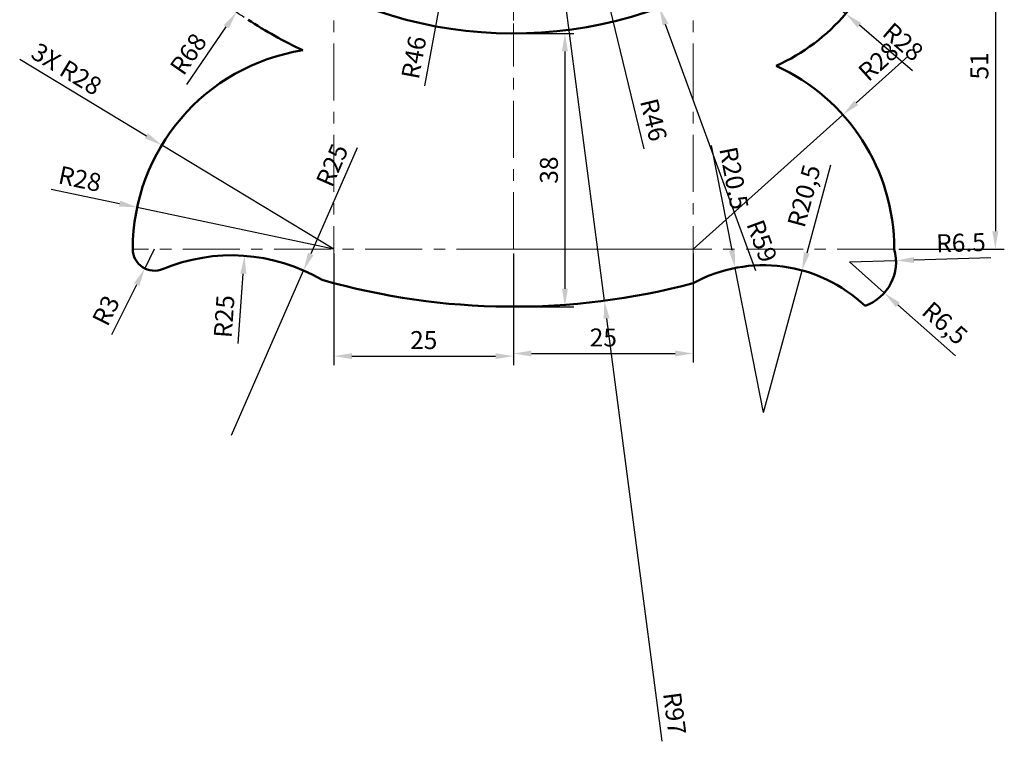
# Model space of a CAD drawing. Units: millimetres. Extents: x 2366 to 2507, y 1526 to 1734.
# Tile 1 of 2: x 2366 to 2503, y 1526 to 1627. Entities that reach past the tile are written whole.
import ezdxf

# ---------------------------------------------------------------- set-up
doc = ezdxf.new("R2010")
doc.units = ezdxf.units.MM
doc.linetypes.add('CENTER', pattern=[50.8, 31.75, -6.35, 6.35, -6.35])
for name, color, linetype, lineweight in [('M-CNTR', 4, 'CENTER', 18), ('M-DIMS', 2, 'Continuous', 25), ('M-OUTL', 7, 'Continuous', 50)]:
    doc.layers.add(name, color=color, linetype=linetype, lineweight=lineweight)
doc.styles.get("Standard").update_dxf_attribs({"font": 'arial.ttf'})
doc.dimstyles.new('ISO-25', dxfattribs={"dimtxt": 2.5, "dimasz": 2.5, "dimexe": 1.25, "dimexo": 0.625, "dimtad": 1, "dimtxsty": 'Standard', "dimcen": 2.5, "dimadec": 0, "dimazin": 0, "dimtfac": 1, "dimtmove": 0, "dimatfit": 3, "dimfxl": 1, "dimarcsym": 0})

# ---------------------------------------------------------------- blocks, each defined once
blk = doc.blocks.new('*D8')
at = {"layer": 'Defpoints', "color": 0, "transparency": 16777216}
for p in [(2492.86, 1645.78), (2488.16, 1594.78), (2502.23, 1594.78)]:
    blk.add_point(p, dxfattribs=at)
at = {"layer": 'M-DIMS', "color": 0, "lineweight": -2, "transparency": 16777216}
for p, q in [((2493.49, 1645.78), (2503.48, 1645.78)), ((2502.23, 1643.28), (2502.23, 1597.28)), ((2488.79, 1594.78), (2503.48, 1594.78))]:
    blk.add_line(p, q, dxfattribs=at)
at = {"layer": 'M-DIMS', "color": 0, "transparency": 16777216}
for points in [[(2501.81, 1643.28), (2502.64, 1643.28), (2502.23, 1645.78)], [(2501.81, 1597.28), (2502.64, 1597.28), (2502.23, 1594.78)]]:
    blk.add_solid(points, dxfattribs=at)
at = {"layer": 'M-DIMS', "color": 0, "transparency": 16777216, "insert": (2500.33, 1620.28), "char_height": 2.5, "attachment_point": 5, "rotation": 90}
blk.add_mtext('51', dxfattribs=at)
blk = doc.blocks.new('*D10')
at = {"layer": 'Defpoints', "color": 0, "transparency": 16777216}
for p in [(2410.16, 1594.78), (2435.16, 1594.78), (2435.16, 1579.9)]:
    blk.add_point(p, dxfattribs=at)
at = {"layer": 'M-DIMS', "color": 0, "lineweight": -2, "transparency": 16777216}
for p, q in [((2410.16, 1594.16), (2410.16, 1578.65)), ((2435.16, 1594.16), (2435.16, 1578.65)), ((2412.66, 1579.9), (2432.66, 1579.9))]:
    blk.add_line(p, q, dxfattribs=at)
at = {"layer": 'M-DIMS', "color": 0, "transparency": 16777216}
for points in [[(2412.66, 1580.32), (2412.66, 1579.49), (2410.16, 1579.9)], [(2432.66, 1580.32), (2432.66, 1579.49), (2435.16, 1579.9)]]:
    blk.add_solid(points, dxfattribs=at)
at = {"layer": 'M-DIMS', "color": 0, "transparency": 16777216, "insert": (2422.66, 1581.81), "char_height": 2.5, "attachment_point": 5}
blk.add_mtext('25', dxfattribs=at)
blk = doc.blocks.new('*D11')
at = {"layer": 'Defpoints', "color": 0, "transparency": 16777216}
for p in [(2435.16, 1594.78), (2460.16, 1594.78), (2460.16, 1580.27)]:
    blk.add_point(p, dxfattribs=at)
at = {"layer": 'M-DIMS', "color": 0, "lineweight": -2, "transparency": 16777216}
for p, q in [((2435.16, 1594.16), (2435.16, 1579.02)), ((2460.16, 1594.16), (2460.16, 1579.02)), ((2437.66, 1580.27), (2457.66, 1580.27))]:
    blk.add_line(p, q, dxfattribs=at)
at = {"layer": 'M-DIMS', "color": 0, "transparency": 16777216}
for points in [[(2437.66, 1580.68), (2437.66, 1579.85), (2435.16, 1580.27)], [(2457.66, 1580.68), (2457.66, 1579.85), (2460.16, 1580.27)]]:
    blk.add_solid(points, dxfattribs=at)
at = {"layer": 'M-DIMS', "color": 0, "transparency": 16777216, "insert": (2447.66, 1582.17), "char_height": 2.5, "attachment_point": 5}
blk.add_mtext('25', dxfattribs=at)
blk = doc.blocks.new('*D12')
at = {"layer": 'Defpoints', "color": 0, "transparency": 16777216}
for p in [(2385.16, 1594.78), (2383.82, 1592.1)]:
    blk.add_point(p, dxfattribs=at)
at = {"layer": 'M-DIMS', "color": 0, "lineweight": -2, "transparency": 16777216}
for p, q in [((2385.16, 1594.78), (2383.82, 1592.1)), ((2379.24, 1582.89), (2382.71, 1589.86))]:
    blk.add_line(p, q, dxfattribs=at)
at = {"layer": 'M-DIMS', "color": 0, "transparency": 16777216}
blk.add_solid([(2382.34, 1590.04), (2383.08, 1589.67), (2383.82, 1592.1)], dxfattribs=at)
at = {"layer": 'M-DIMS', "color": 0, "transparency": 16777216, "insert": (2378.71, 1586.11), "char_height": 2.5, "attachment_point": 5, "rotation": 63.5125}
blk.add_mtext('R3', dxfattribs=at)
blk = doc.blocks.new('*D13')
at = {"layer": 'Defpoints', "color": 0, "transparency": 16777216}
for p in [(2397.73, 1593.86), (2395.91, 1568.93)]:
    blk.add_point(p, dxfattribs=at)
at = {"layer": 'M-DIMS', "color": 0, "lineweight": -2, "transparency": 16777216}
blk.add_line((2396.84, 1581.65), (2397.54, 1591.37), dxfattribs=at)
at = {"layer": 'M-DIMS', "color": 0, "transparency": 16777216}
blk.add_solid([(2397.13, 1591.4), (2397.96, 1591.34), (2397.73, 1593.86)], dxfattribs=at)
at = {"layer": 'M-DIMS', "color": 0, "transparency": 16777216, "insert": (2395.2, 1585.4), "char_height": 2.5, "attachment_point": 5, "rotation": 85.8254}
blk.add_mtext('R25', dxfattribs=at)
blk = doc.blocks.new('*D14')
at = {"layer": 'Defpoints', "color": 0, "transparency": 16777216}
for p in [(2475.32, 1591.83), (2469.95, 1572.04)]:
    blk.add_point(p, dxfattribs=at)
at = {"layer": 'M-DIMS', "color": 0, "lineweight": -2, "transparency": 16777216}
for p, q in [((2479.29, 1606.45), (2475.97, 1594.24)), ((2469.95, 1572.04), (2475.32, 1591.83))]:
    blk.add_line(p, q, dxfattribs=at)
at = {"layer": 'M-DIMS', "color": 0, "transparency": 16777216}
blk.add_solid([(2475.57, 1594.35), (2476.37, 1594.13), (2475.32, 1591.83)], dxfattribs=at)
at = {"layer": 'M-DIMS', "color": 0, "transparency": 16777216, "insert": (2475.9, 1602.11), "char_height": 2.5, "attachment_point": 5, "rotation": 74.8103}
blk.add_mtext('R20,5', dxfattribs=at)
blk = doc.blocks.new('*D15')
at = {"layer": 'Defpoints', "color": 0, "transparency": 16777216}
for p in [(2435.16, 1624.78), (2435.16, 1586.78), (2442.31, 1586.78)]:
    blk.add_point(p, dxfattribs=at)
at = {"layer": 'M-DIMS', "color": 0, "lineweight": -2, "transparency": 16777216}
for p, q in [((2435.79, 1624.78), (2443.56, 1624.78)), ((2442.31, 1622.28), (2442.31, 1589.28)), ((2435.79, 1586.78), (2443.56, 1586.78))]:
    blk.add_line(p, q, dxfattribs=at)
at = {"layer": 'M-DIMS', "color": 0, "transparency": 16777216}
for points in [[(2441.9, 1622.28), (2442.73, 1622.28), (2442.31, 1624.78)], [(2441.9, 1589.28), (2442.73, 1589.28), (2442.31, 1586.78)]]:
    blk.add_solid(points, dxfattribs=at)
at = {"layer": 'M-DIMS', "color": 0, "transparency": 16777216, "insert": (2440.41, 1605.78), "char_height": 2.5, "attachment_point": 5, "rotation": 90}
blk.add_mtext('38', dxfattribs=at)
blk = doc.blocks.new('*D16')
at = {"layer": 'Defpoints', "color": 0, "transparency": 16777216}
for p in [(2481.01, 1613.47), (2460.16, 1594.78)]:
    blk.add_point(p, dxfattribs=at)
at = {"layer": 'M-DIMS', "color": 0, "lineweight": -2, "transparency": 16777216}
for p, q in [((2490.11, 1621.64), (2482.87, 1615.14)), ((2460.16, 1594.78), (2481.01, 1613.47))]:
    blk.add_line(p, q, dxfattribs=at)
at = {"layer": 'M-DIMS', "color": 0, "transparency": 16777216}
blk.add_solid([(2482.59, 1615.45), (2483.15, 1614.83), (2481.01, 1613.47)], dxfattribs=at)
at = {"layer": 'M-DIMS', "color": 0, "transparency": 16777216, "insert": (2486.15, 1620.64), "char_height": 2.5, "attachment_point": 5, "rotation": 41.8846}
blk.add_mtext('R28', dxfattribs=at)
blk = doc.blocks.new('*D17')
at = {"layer": 'Defpoints', "color": 0, "transparency": 16777216}
for p in [(2481.91, 1593.01), (2486.77, 1588.7)]:
    blk.add_point(p, dxfattribs=at)
at = {"layer": 'M-DIMS', "color": 0, "lineweight": -2, "transparency": 16777216}
for p, q in [((2481.91, 1593.01), (2486.77, 1588.7)), ((2496.66, 1579.94), (2488.64, 1587.04))]:
    blk.add_line(p, q, dxfattribs=at)
at = {"layer": 'M-DIMS', "color": 0, "transparency": 16777216}
blk.add_solid([(2488.92, 1587.35), (2488.37, 1586.73), (2486.77, 1588.7)], dxfattribs=at)
at = {"layer": 'M-DIMS', "color": 0, "transparency": 16777216, "insert": (2495, 1584.25), "char_height": 2.5, "attachment_point": 5, "rotation": 318.4548}
blk.add_mtext('R6,5', dxfattribs=at)
blk = doc.blocks.new('*D18')
at = {"layer": 'Defpoints', "color": 0, "transparency": 16777216}
for p in [(2435.16, 1683.78), (2426.73, 1638.56)]:
    blk.add_point(p, dxfattribs=at)
at = {"layer": 'M-DIMS', "color": 0, "lineweight": -2, "transparency": 16777216}
for p, q in [((2435.16, 1683.78), (2426.73, 1638.56)), ((2422.8, 1617.49), (2426.27, 1636.1))]:
    blk.add_line(p, q, dxfattribs=at)
at = {"layer": 'M-DIMS', "color": 0, "transparency": 16777216}
blk.add_solid([(2425.86, 1636.18), (2426.68, 1636.03), (2426.73, 1638.56)], dxfattribs=at)
at = {"layer": 'M-DIMS', "color": 0, "transparency": 16777216, "insert": (2421.6, 1621.39), "char_height": 2.5, "attachment_point": 5, "rotation": 79.4409}
blk.add_mtext('R46', dxfattribs=at)
blk = doc.blocks.new('*D19')
at = {"layer": 'Defpoints', "color": 0, "transparency": 16777216}
for p in [(2435.16, 1683.78), (2396.6, 1627.77)]:
    blk.add_point(p, dxfattribs=at)
at = {"layer": 'M-DIMS', "color": 0, "lineweight": -2, "transparency": 16777216}
for p, q in [((2435.16, 1683.78), (2396.6, 1627.77)), ((2389.67, 1617.7), (2395.18, 1625.71))]:
    blk.add_line(p, q, dxfattribs=at)
blk.add_arc((2435.16, 1683.78), 68, 234.401, 236.5526, dxfattribs=at)
at = {"layer": 'M-DIMS', "color": 0, "transparency": 16777216}
blk.add_solid([(2394.84, 1625.95), (2395.53, 1625.48), (2396.6, 1627.77)], dxfattribs=at)
at = {"layer": 'M-DIMS', "color": 0, "transparency": 16777216, "insert": (2390.15, 1621.75), "char_height": 2.5, "attachment_point": 5, "rotation": 55.4543}
blk.add_mtext('R68', dxfattribs=at)
blk = doc.blocks.new('*D23')
at = {"layer": 'Defpoints', "color": 0, "transparency": 16777216}
for p in [(2382.77, 1600.6), (2410.16, 1594.78)]:
    blk.add_point(p, dxfattribs=at)
at = {"layer": 'M-DIMS', "color": 0, "lineweight": -2, "transparency": 16777216}
for p, q in [((2370.81, 1603.14), (2380.33, 1601.12)), ((2410.16, 1594.78), (2382.77, 1600.6))]:
    blk.add_line(p, q, dxfattribs=at)
at = {"layer": 'M-DIMS', "color": 0, "transparency": 16777216}
blk.add_solid([(2380.41, 1601.53), (2380.24, 1600.71), (2382.77, 1600.6)], dxfattribs=at)
at = {"layer": 'M-DIMS', "color": 0, "transparency": 16777216, "insert": (2374.74, 1604.25), "char_height": 2.5, "attachment_point": 5, "rotation": 348.0092}
blk.add_mtext('R28', dxfattribs=at)
blk = doc.blocks.new('*D24')
at = {"layer": 'Defpoints', "color": 0, "transparency": 16777216}
for p in [(2460.16, 1645.78), (2481.41, 1627.54)]:
    blk.add_point(p, dxfattribs=at)
at = {"layer": 'M-DIMS', "color": 0, "lineweight": -2, "transparency": 16777216}
for p, q in [((2460.16, 1645.78), (2481.41, 1627.54)), ((2490.69, 1619.58), (2483.3, 1625.92))]:
    blk.add_line(p, q, dxfattribs=at)
at = {"layer": 'M-DIMS', "color": 0, "transparency": 16777216}
blk.add_solid([(2483.58, 1626.23), (2483.03, 1625.6), (2481.41, 1627.54)], dxfattribs=at)
at = {"layer": 'M-DIMS', "color": 0, "transparency": 16777216, "insert": (2489.18, 1623.38), "char_height": 2.5, "attachment_point": 5, "rotation": 319.3585}
blk.add_mtext('R28', dxfattribs=at)
blk = doc.blocks.new('*D38')
at = {"layer": 'Defpoints', "color": 0, "transparency": 16777216}
for p in [(2435.16, 1683.78), (2447.8, 1587.61)]:
    blk.add_point(p, dxfattribs=at)
at = {"layer": 'M-DIMS', "color": 0, "lineweight": -2, "transparency": 16777216}
for p, q in [((2435.16, 1683.78), (2447.8, 1587.61)), ((2455.85, 1526.32), (2448.13, 1585.13))]:
    blk.add_line(p, q, dxfattribs=at)
at = {"layer": 'M-DIMS', "color": 0, "transparency": 16777216}
blk.add_solid([(2448.54, 1585.18), (2447.71, 1585.08), (2447.8, 1587.61)], dxfattribs=at)
at = {"layer": 'M-DIMS', "color": 0, "transparency": 16777216, "insert": (2457.27, 1530.15), "char_height": 2.5, "attachment_point": 5, "rotation": 277.4868}
blk.add_mtext('R97', dxfattribs=at)
blk = doc.blocks.new('*D39')
at = {"layer": 'Defpoints', "color": 0, "transparency": 16777216}
for p in [(2435.16, 1683.78), (2455.46, 1628.38)]:
    blk.add_point(p, dxfattribs=at)
at = {"layer": 'M-DIMS', "color": 0, "lineweight": -2, "transparency": 16777216}
for p, q in [((2435.16, 1683.78), (2455.46, 1628.38)), ((2468.89, 1591.75), (2456.32, 1626.04))]:
    blk.add_line(p, q, dxfattribs=at)
at = {"layer": 'M-DIMS', "color": 0, "transparency": 16777216}
blk.add_solid([(2456.71, 1626.18), (2455.93, 1625.89), (2455.46, 1628.38)], dxfattribs=at)
at = {"layer": 'M-DIMS', "color": 0, "transparency": 16777216, "insert": (2469.43, 1595.8), "char_height": 2.5, "attachment_point": 5, "rotation": 290.1259}
blk.add_mtext('R59', dxfattribs=at)
blk = doc.blocks.new('*D40')
at = {"layer": 'Defpoints', "color": 0, "transparency": 16777216}
for p in [(2435.16, 1683.78), (2446, 1639.08)]:
    blk.add_point(p, dxfattribs=at)
at = {"layer": 'M-DIMS', "color": 0, "lineweight": -2, "transparency": 16777216}
for p, q in [((2435.16, 1683.78), (2446, 1639.08)), ((2453.36, 1608.74), (2446.59, 1636.65))]:
    blk.add_line(p, q, dxfattribs=at)
at = {"layer": 'M-DIMS', "color": 0, "transparency": 16777216}
blk.add_solid([(2446.99, 1636.75), (2446.19, 1636.55), (2446, 1639.08)], dxfattribs=at)
at = {"layer": 'M-DIMS', "color": 0, "transparency": 16777216, "insert": (2454.35, 1612.7), "char_height": 2.5, "attachment_point": 5, "rotation": 283.6294}
blk.add_mtext('R46', dxfattribs=at)
blk = doc.blocks.new('*D42')
at = {"layer": 'Defpoints', "color": 0, "transparency": 16777216}
for p in [(2386.19, 1609.25), (2410.16, 1594.78)]:
    blk.add_point(p, dxfattribs=at)
at = {"layer": 'M-DIMS', "color": 0, "lineweight": -2, "transparency": 16777216}
for p, q in [((2366.42, 1621.2), (2384.05, 1610.55)), ((2410.16, 1594.78), (2386.19, 1609.25))]:
    blk.add_line(p, q, dxfattribs=at)
at = {"layer": 'M-DIMS', "color": 0, "transparency": 16777216}
blk.add_solid([(2384.27, 1610.9), (2383.84, 1610.19), (2386.19, 1609.25)], dxfattribs=at)
at = {"layer": 'M-DIMS', "color": 0, "transparency": 16777216, "insert": (2372.79, 1619.57), "char_height": 2.5, "attachment_point": 5, "rotation": 328.8746}
blk.add_mtext('3X R28', dxfattribs=at)
blk = doc.blocks.new('*D47')
at = {"layer": 'Defpoints', "color": 0, "transparency": 16777216}
for p in [(2481.91, 1593.01), (2488.4, 1593.2)]:
    blk.add_point(p, dxfattribs=at)
at = {"layer": 'M-DIMS', "color": 0, "lineweight": -2, "transparency": 16777216}
for p, q in [((2481.91, 1593.01), (2488.4, 1593.2)), ((2501.61, 1593.58), (2490.9, 1593.27))]:
    blk.add_line(p, q, dxfattribs=at)
at = {"layer": 'M-DIMS', "color": 0, "transparency": 16777216}
blk.add_solid([(2490.89, 1593.69), (2490.92, 1592.85), (2488.4, 1593.2)], dxfattribs=at)
at = {"layer": 'M-DIMS', "color": 0, "transparency": 16777216, "insert": (2497.45, 1595.36), "char_height": 2.5, "attachment_point": 5, "rotation": 1.6522}
blk.add_mtext('R6.5', dxfattribs=at)
blk = doc.blocks.new('*D49')
at = {"layer": 'Defpoints', "color": 0, "transparency": 16777216}
for p in [(2405.93, 1591.83), (2395.91, 1568.93)]:
    blk.add_point(p, dxfattribs=at)
at = {"layer": 'M-DIMS', "color": 0, "lineweight": -2, "transparency": 16777216}
for p, q in [((2413.4, 1608.89), (2406.94, 1594.12)), ((2395.91, 1568.93), (2405.93, 1591.83))]:
    blk.add_line(p, q, dxfattribs=at)
at = {"layer": 'M-DIMS', "color": 0, "transparency": 16777216}
blk.add_solid([(2406.55, 1594.28), (2407.32, 1593.95), (2405.93, 1591.83)], dxfattribs=at)
at = {"layer": 'M-DIMS', "color": 0, "transparency": 16777216, "insert": (2410.21, 1606.33), "char_height": 2.5, "attachment_point": 5, "rotation": 66.3569}
blk.add_mtext('R25', dxfattribs=at)
blk = doc.blocks.new('*D50')
at = {"layer": 'Defpoints', "color": 0, "transparency": 16777216}
for p in [(2466.02, 1592.16), (2469.95, 1572.04)]:
    blk.add_point(p, dxfattribs=at)
at = {"layer": 'M-DIMS', "color": 0, "lineweight": -2, "transparency": 16777216}
for p, q in [((2462.69, 1609.22), (2465.54, 1594.62)), ((2469.95, 1572.04), (2466.02, 1592.16))]:
    blk.add_line(p, q, dxfattribs=at)
at = {"layer": 'M-DIMS', "color": 0, "transparency": 16777216}
blk.add_solid([(2465.95, 1594.7), (2465.13, 1594.54), (2466.02, 1592.16)], dxfattribs=at)
at = {"layer": 'M-DIMS', "color": 0, "transparency": 16777216, "insert": (2465.53, 1604.6), "char_height": 2.5, "attachment_point": 5, "rotation": 281.0506}
blk.add_mtext('R20.5', dxfattribs=at)

msp = doc.modelspace()

# ---------------------------------------------------------------- linework, layer by layer
at = {"layer": 'M-CNTR', "ltscale": 0.25}
for p, q in [((2435.161, 1675.781), (2435.161, 1626.165)), ((2410.161, 1590.058), (2410.161, 1645.168)), ((2460.161, 1590.058), (2460.161, 1645.168)), ((2435.161, 1594.781), (2435.161, 1626.165)), ((2435.161, 1594.781), (2382.161, 1594.781)), ((2488.161, 1594.781), (2435.161, 1594.781)), ((2435.161, 1594.781), (2460.161, 1594.781))]:
    msp.add_line(p, q, dxfattribs=at)
at = {"layer": 'M-OUTL'}
for centre, radius, start, end in [((2460.161, 1645.781), 28, 294.39575, 344.32119), ((2435.161, 1683.781), 59, 236.4813, 302.92073), ((2435.161, 1683.781), 68, 237.07927, 244.4299), ((2410.161, 1594.781), 28, 98.93714, 180), ((2460.161, 1594.781), 28, 0, 65.60425), ((2385.161, 1594.781), 3, 180, 293.3445), ((2481.907, 1593.01), 6.5, 289.59014, 15.81031), ((2395.907, 1568.925), 25, 59.70834, 112.66117), ((2469.946, 1572.044), 20.5, 46.38733, 118.50969), ((2435.161, 1683.781), 97, 254.05688, 284.93553)]:
    msp.add_arc(centre, radius, start, end, dxfattribs=at)

# ---------------------------------------------------------------- dimensions: what is measured, and where the dimension line sits
at = {"layer": 'M-DIMS'}
for center, mpoint, override, picture, middle in [((2435.161, 1683.781), (2396.601, 1627.771), {"dimclrd": 0, "dimclre": 0, "dimclrt": 0}, '*D19', (2390.15, 1621.754)), ((2460.161, 1645.781), (2481.408, 1627.544), {"dimclrd": 0, "dimclre": 0, "dimclrt": 0}, '*D24', (2489.183, 1623.376)), ((2460.161, 1594.781), (2481.007, 1613.475), {"dimclrd": 0, "dimclre": 0, "dimclrt": 0}, '*D16', (2486.151, 1620.642)), ((2410.161, 1594.781), (2382.772, 1600.598), {"dimclrd": 0, "dimclre": 0, "dimclrt": 0}, '*D23', (2374.741, 1604.248)), ((2469.946, 1572.044), (2475.317, 1591.828), {"dimclrd": 0, "dimclre": 0, "dimclrt": 0}, '*D14', (2475.905, 1602.111)), ((2481.907, 1593.01), (2488.405, 1593.198), {"dimdec": 1, "dimlfac": 1, "dimrnd": 0, "dimzin": 0, "dimdsep": 46, "dimlunit": 2}, '*D47', (2497.452, 1595.361)), ((2385.161, 1594.781), (2383.823, 1592.096), {"dimclrd": 0, "dimclre": 0, "dimclrt": 0}, '*D12', (2378.713, 1586.106)), ((2481.907, 1593.01), (2486.772, 1588.699), {"dimclrd": 0, "dimclre": 0, "dimclrt": 0}, '*D17', (2494.999, 1584.252))]:
    dim = msp.add_radius_dim(center=center, mpoint=mpoint, dimstyle='ISO-25', override=override, dxfattribs=at)
    dim.commit()
    dim.dimension.update_dxf_attribs({"geometry": picture, "text_midpoint": middle})
for center, mpoint, override, picture, middle in [((2435.161, 1683.781), (2426.732, 1638.56), {"dimclrd": 0, "dimclre": 0, "dimclrt": 0}, '*D18', (2423.466, 1621.04)), ((2435.161, 1683.781), (2447.8, 1587.608), {"dimdec": 0, "dimlfac": 1, "dimrnd": 0, "dimzin": 0, "dimdsep": 46, "dimlunit": 2}, '*D38', (2455.384, 1529.904)), ((2435.161, 1683.781), (2455.462, 1628.384), {"dimdec": 0, "dimlfac": 1, "dimrnd": 0, "dimzin": 0, "dimdsep": 46, "dimlunit": 2}, '*D39', (2467.643, 1595.145)), ((2435.161, 1683.781), (2446.001, 1639.076), {"dimdec": 0, "dimlfac": 1, "dimrnd": 0, "dimzin": 0, "dimdsep": 46, "dimlunit": 2}, '*D40', (2452.505, 1612.254)), ((2395.907, 1568.925), (2405.933, 1591.827), {"dimdec": 0, "dimlfac": 1, "dimrnd": 0, "dimzin": 0, "dimdsep": 46, "dimlunit": 2}, '*D49', (2411.949, 1605.568)), ((2469.946, 1572.044), (2466.017, 1592.164), {"dimdec": 1, "dimlfac": 1, "dimrnd": 0, "dimzin": 0, "dimdsep": 46, "dimlunit": 2}, '*D50', (2463.659, 1604.236)), ((2395.907, 1568.925), (2397.727, 1593.859), {"dimclrd": 0, "dimclre": 0, "dimclrt": 0}, '*D13', (2397.099, 1585.261))]:
    dim = msp.add_radius_dim(center=center, mpoint=mpoint, dimstyle='ISO-25', override=override, dxfattribs=at)
    dim.commit()
    dim.dimension.update_dxf_attribs({"geometry": picture, "text_midpoint": middle, "dimtype": 164})
for base, p1, p2, picture, middle in [((2502.227, 1594.781), (2492.863, 1645.781), (2488.161, 1594.781), '*D8', (2500.325, 1620.281)), ((2442.314, 1586.781), (2435.161, 1624.781), (2435.161, 1586.781), '*D15', (2440.411, 1605.781))]:
    dim = msp.add_linear_dim(base=base, p1=p1, p2=p2, angle=90, dimstyle='ISO-25', override={"dimclrd": 0, "dimclre": 0, "dimclrt": 0}, dxfattribs=at)
    dim.commit()
    dim.dimension.update_dxf_attribs({"geometry": picture, "text_midpoint": middle})
dim = msp.add_radius_dim(center=(2410.161, 1594.781), mpoint=(2386.192, 1609.255), text='3X <>', dimstyle='ISO-25', override={"dimdec": 0, "dimlfac": 1, "dimrnd": 0, "dimzin": 0, "dimdsep": 46, "dimlunit": 2}, dxfattribs=at)
dim.commit()
dim.dimension.update_dxf_attribs({"geometry": '*D42', "text_midpoint": (2371.811, 1617.939), "dimtype": 164})
for base, p1, p2, picture, middle in [((2435.161, 1579.904), (2410.161, 1594.781), (2435.161, 1594.781), '*D10', (2422.661, 1581.805)), ((2460.161, 1580.267), (2435.161, 1594.781), (2460.161, 1594.781), '*D11', (2447.661, 1582.169))]:
    dim = msp.add_linear_dim(base=base, p1=p1, p2=p2, dimstyle='ISO-25', override={"dimclrd": 0, "dimclre": 0, "dimclrt": 0}, dxfattribs=at)
    dim.commit()
    dim.dimension.update_dxf_attribs({"geometry": picture, "text_midpoint": middle})

doc.saveas('drawing.dxf')
